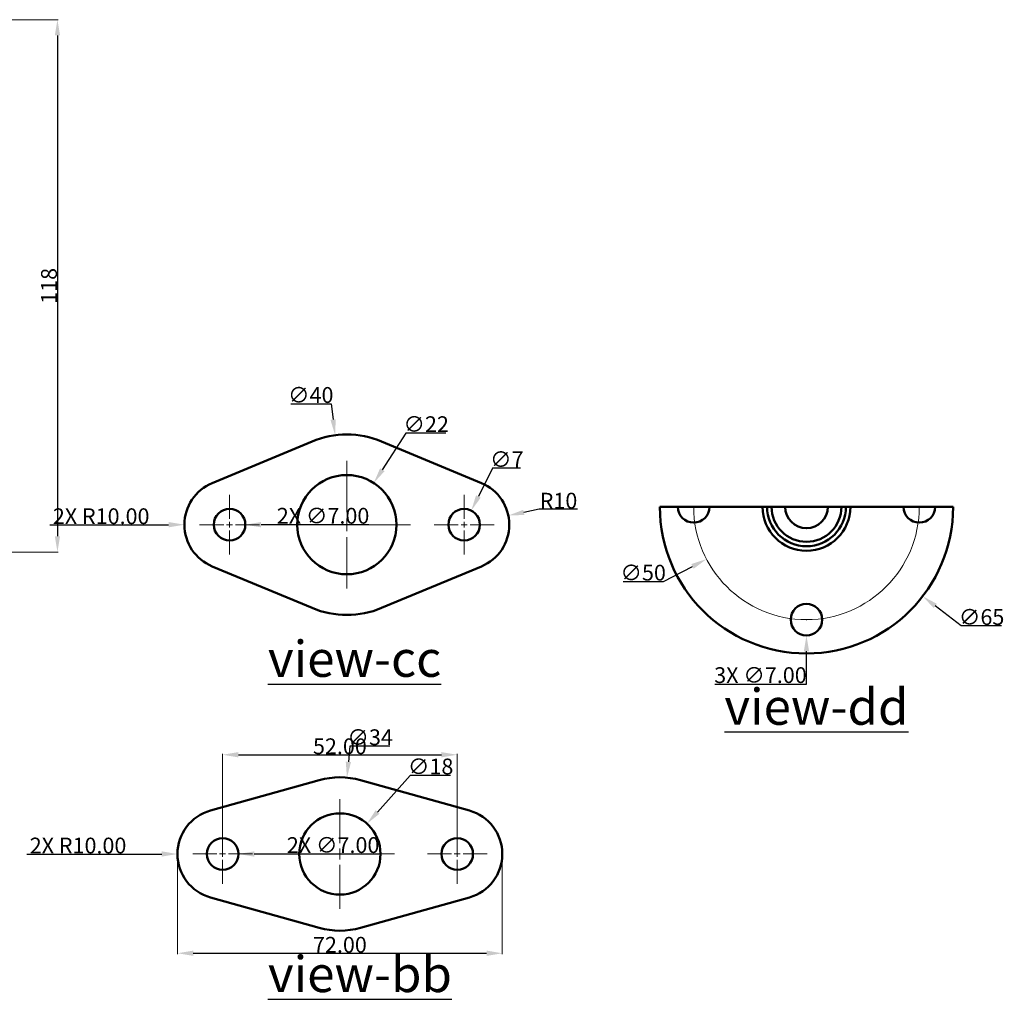
# Model space of a CAD drawing. Units: millimetres. Extents: x 75 to 489, y 21 to 350.
# Tile 5 of 5: x 271 to 489, y 110 to 327. Entities that reach past the tile are written whole.
import ezdxf

# ---------------------------------------------------------------- set-up
doc = ezdxf.new("R2010")
doc.units = ezdxf.units.MM
doc.header["$MEASUREMENT"] = 0
doc.linetypes.add('CENTER', pattern=[50.8, 31.75, -6.35, 6.35, -6.35])
for name, color, linetype, lineweight in [('M-CNTR', 1, 'CENTER', 18), ('M-CONS', 9, 'Continuous', 13), ('M-DIMS', 2, 'Continuous', 25), ('M-OUTL', 7, 'Continuous', 50), ('M-TEXT', 7, 'Continuous', 25)]:
    doc.layers.add(name, color=color, linetype=linetype, lineweight=lineweight)
doc.styles.get("Standard").update_dxf_attribs({"font": 'arial.ttf'})
doc.dimstyles.get("Standard").update_dxf_attribs({"dimtxt": 3.5, "dimasz": 3.5, "dimexe": 0.18, "dimexo": 0.0625, "dimgap": 0.09, "dimtad": 1, "dimtoh": 1, "dimdec": 0, "dimzin": 0, "dimdsep": 46, "dimtxsty": 'Standard', "dimcen": 0.09, "dimclrd": 2, "dimclre": 251, "dimadec": 0, "dimazin": 0, "dimtfac": 1, "dimtdec": 0, "dimtofl": 0, "dimtmove": 0, "dimatfit": 3, "dimfxl": 1, "dimtolj": 1, "dimtzin": 0, "dimlwe": 5, "dimarcsym": 0})

# ---------------------------------------------------------------- blocks, each defined once
blk = doc.blocks.new('*U1')
at = {"layer": 'M-CNTR', "color": 0, "transparency": 16777216}
for p, q in [((0, 1.3), (0, 6.62)), ((-6.62, 0), (-1.3, 0)), ((1.3, 0), (6.62, 0)), ((0, -6.62), (0, -1.3))]:
    blk.add_line(p, q, dxfattribs=at)
at = {"layer": 'M-CNTR', "color": 0, "linetype": 'Continuous', "transparency": 16777216}
for p, q in [((-0.65, 0), (0.65, 0)), ((0, -0.65), (0, 0.65))]:
    blk.add_line(p, q, dxfattribs=at)
blk = doc.blocks.new('*U2')
at = {"layer": 'M-CNTR', "color": 0, "transparency": 16777216}
for p, q in [((0, 1.3), (0, 6.62)), ((-6.62, 0), (-1.3, 0)), ((1.3, 0), (6.62, 0)), ((0, -6.62), (0, -1.3))]:
    blk.add_line(p, q, dxfattribs=at)
at = {"layer": 'M-CNTR', "color": 0, "linetype": 'Continuous', "transparency": 16777216}
for p, q in [((-0.65, 0), (0.65, 0)), ((0, -0.65), (0, 0.65))]:
    blk.add_line(p, q, dxfattribs=at)
blk = doc.blocks.new('*U3')
at = {"layer": 'M-CNTR', "color": 0, "transparency": 16777216}
for p, q in [((0, 2.8), (0, 14.12)), ((-14.12, 0), (-2.8, 0)), ((2.8, 0), (14.12, 0)), ((0, -14.12), (0, -2.8))]:
    blk.add_line(p, q, dxfattribs=at)
at = {"layer": 'M-CNTR', "color": 0, "linetype": 'Continuous', "transparency": 16777216}
for p, q in [((-1.4, 0), (1.4, 0)), ((0, -1.4), (0, 1.4))]:
    blk.add_line(p, q, dxfattribs=at)
blk = doc.blocks.new('*D4')
at = {"layer": 'Defpoints', "color": 0, "transparency": 16777216}
for p in [(349.6, 224.66), (337.68, 206.17)]:
    blk.add_point(p, dxfattribs=at)
at = {"layer": 'M-DIMS', "color": 0, "lineweight": -2, "transparency": 16777216}
for p, q in [((356.74, 235.71), (351.5, 227.6)), ((365.61, 235.71), (356.74, 235.71))]:
    blk.add_line(p, q, dxfattribs=at)
at = {"layer": 'M-DIMS', "color": 0, "lineweight": 5, "transparency": 16777216}
for p, q in [((343.55, 215.41), (343.73, 215.41)), ((343.64, 215.32), (343.64, 215.5))]:
    blk.add_line(p, q, dxfattribs=at)
at = {"layer": 'M-DIMS', "color": 0, "transparency": 16777216}
blk.add_solid([(351.01, 227.91), (351.99, 227.28), (349.6, 224.66)], dxfattribs=at)
at = {"layer": 'M-DIMS', "color": 0, "transparency": 16777216, "insert": (361.22, 237.69), "char_height": 3.5, "attachment_point": 5}
blk.add_mtext('\\A1;∅22', dxfattribs=at)
blk = doc.blocks.new('*D5')
at = {"layer": 'Defpoints', "color": 0, "transparency": 16777216}
for p in [(341.05, 235.24), (346.23, 195.58)]:
    blk.add_point(p, dxfattribs=at)
at = {"layer": 'M-DIMS', "color": 0, "lineweight": -2, "transparency": 16777216}
for p, q in [((331.24, 242.18), (340.14, 242.18)), ((340.14, 242.18), (340.59, 238.71))]:
    blk.add_line(p, q, dxfattribs=at)
at = {"layer": 'M-DIMS', "color": 0, "lineweight": 5, "transparency": 16777216}
for p, q in [((343.55, 215.41), (343.73, 215.41)), ((343.64, 215.32), (343.64, 215.5))]:
    blk.add_line(p, q, dxfattribs=at)
at = {"layer": 'M-DIMS', "color": 0, "transparency": 16777216}
blk.add_solid([(341.17, 238.79), (340.01, 238.64), (341.05, 235.24)], dxfattribs=at)
at = {"layer": 'M-DIMS', "color": 0, "transparency": 16777216, "insert": (335.64, 244.16), "char_height": 3.5, "attachment_point": 5}
blk.add_mtext('\\A1;∅40', dxfattribs=at)
blk = doc.blocks.new('*D6')
at = {"layer": 'Defpoints', "color": 0, "transparency": 16777216}
for p in [(371.22, 218.54), (368.06, 212.29)]:
    blk.add_point(p, dxfattribs=at)
at = {"layer": 'M-DIMS', "color": 0, "lineweight": -2, "transparency": 16777216}
for p, q in [((375.95, 227.93), (372.79, 221.66)), ((382.14, 227.93), (375.95, 227.93))]:
    blk.add_line(p, q, dxfattribs=at)
at = {"layer": 'M-DIMS', "color": 0, "lineweight": 5, "transparency": 16777216}
for p, q in [((369.55, 215.41), (369.73, 215.41)), ((369.64, 215.32), (369.64, 215.5))]:
    blk.add_line(p, q, dxfattribs=at)
at = {"layer": 'M-DIMS', "color": 0, "transparency": 16777216}
blk.add_solid([(372.27, 221.93), (373.31, 221.4), (371.22, 218.54)], dxfattribs=at)
at = {"layer": 'M-DIMS', "color": 0, "transparency": 16777216, "insert": (379.09, 229.9), "char_height": 3.5, "attachment_point": 5}
blk.add_mtext('\\A1;∅7', dxfattribs=at)
blk = doc.blocks.new('*D7')
at = {"layer": 'Defpoints', "color": 0, "transparency": 16777216}
for p in [(379.43, 217.44), (369.64, 215.41)]:
    blk.add_point(p, dxfattribs=at)
at = {"layer": 'M-DIMS', "color": 0, "lineweight": -2, "transparency": 16777216}
for p, q in [((386.29, 218.85), (382.86, 218.14)), ((394.73, 218.85), (386.29, 218.85))]:
    blk.add_line(p, q, dxfattribs=at)
at = {"layer": 'M-DIMS', "color": 0, "lineweight": 5, "transparency": 16777216}
for p, q in [((369.55, 215.41), (369.73, 215.41)), ((369.64, 215.32), (369.64, 215.5))]:
    blk.add_line(p, q, dxfattribs=at)
at = {"layer": 'M-DIMS', "color": 0, "transparency": 16777216}
blk.add_solid([(382.74, 218.71), (382.98, 217.57), (379.43, 217.44)], dxfattribs=at)
at = {"layer": 'M-DIMS', "color": 0, "transparency": 16777216, "insert": (390.55, 220.73), "char_height": 3.5, "attachment_point": 5}
blk.add_mtext('\\A1;R10', dxfattribs=at)
blk = doc.blocks.new('*U8')
at = {"layer": 'M-CNTR', "color": 0, "transparency": 16777216}
for p, q in [((0, 1.3), (0, 6.62)), ((-6.62, 0), (-1.3, 0)), ((1.3, 0), (6.62, 0)), ((0, -6.62), (0, -1.3))]:
    blk.add_line(p, q, dxfattribs=at)
at = {"layer": 'M-CNTR', "color": 0, "linetype": 'Continuous', "transparency": 16777216}
for p, q in [((-0.65, 0), (0.65, 0)), ((0, -0.65), (0, 0.65))]:
    blk.add_line(p, q, dxfattribs=at)
blk = doc.blocks.new('*U9')
at = {"layer": 'M-CNTR', "color": 0, "transparency": 16777216}
for p, q in [((0, 2.4), (0, 12.12)), ((-12.12, 0), (-2.4, 0)), ((2.4, 0), (12.12, 0)), ((0, -12.12), (0, -2.4))]:
    blk.add_line(p, q, dxfattribs=at)
at = {"layer": 'M-CNTR', "color": 0, "linetype": 'Continuous', "transparency": 16777216}
for p, q in [((-1.2, 0), (1.2, 0)), ((0, -1.2), (0, 1.2))]:
    blk.add_line(p, q, dxfattribs=at)
blk = doc.blocks.new('*U10')
at = {"layer": 'M-CNTR', "color": 0, "transparency": 16777216}
for p, q in [((0, 1.3), (0, 6.62)), ((-6.62, 0), (-1.3, 0)), ((1.3, 0), (6.62, 0)), ((0, -6.62), (0, -1.3))]:
    blk.add_line(p, q, dxfattribs=at)
at = {"layer": 'M-CNTR', "color": 0, "linetype": 'Continuous', "transparency": 16777216}
for p, q in [((-0.65, 0), (0.65, 0)), ((0, -0.65), (0, 0.65))]:
    blk.add_line(p, q, dxfattribs=at)
blk = doc.blocks.new('*D11')
at = {"layer": 'Defpoints', "color": 0, "transparency": 16777216}
for p in [(343.66, 159.35), (340.53, 125.5)]:
    blk.add_point(p, dxfattribs=at)
at = {"layer": 'M-DIMS', "color": 0, "lineweight": -2, "transparency": 16777216}
for p, q in [((344.31, 166.32), (343.98, 162.84)), ((353.2, 166.32), (344.31, 166.32))]:
    blk.add_line(p, q, dxfattribs=at)
at = {"layer": 'M-DIMS', "color": 0, "lineweight": 5, "transparency": 16777216}
for p, q in [((342.01, 142.42), (342.19, 142.42)), ((342.1, 142.33), (342.1, 142.51))]:
    blk.add_line(p, q, dxfattribs=at)
at = {"layer": 'M-DIMS', "color": 0, "transparency": 16777216}
blk.add_solid([(343.4, 162.89), (344.56, 162.78), (343.66, 159.35)], dxfattribs=at)
at = {"layer": 'M-DIMS', "color": 0, "transparency": 16777216, "insert": (348.8, 168.3), "char_height": 3.5, "attachment_point": 5}
blk.add_mtext('\\A1;∅34', dxfattribs=at)
blk = doc.blocks.new('*D12')
at = {"layer": 'Defpoints', "color": 0, "transparency": 16777216}
for p in [(348.1, 149.13), (336.09, 135.72)]:
    blk.add_point(p, dxfattribs=at)
at = {"layer": 'M-DIMS', "color": 0, "lineweight": -2, "transparency": 16777216}
for p, q in [((357.71, 159.84), (350.44, 151.73)), ((366.63, 159.84), (357.71, 159.84))]:
    blk.add_line(p, q, dxfattribs=at)
at = {"layer": 'M-DIMS', "color": 0, "lineweight": 5, "transparency": 16777216}
for p, q in [((342.01, 142.42), (342.19, 142.42)), ((342.1, 142.33), (342.1, 142.51))]:
    blk.add_line(p, q, dxfattribs=at)
at = {"layer": 'M-DIMS', "color": 0, "transparency": 16777216}
blk.add_solid([(350.01, 152.12), (350.87, 151.34), (348.1, 149.13)], dxfattribs=at)
at = {"layer": 'M-DIMS', "color": 0, "transparency": 16777216, "insert": (362.21, 161.82), "char_height": 3.5, "attachment_point": 5}
blk.add_mtext('\\A1;∅18', dxfattribs=at)
blk = doc.blocks.new('*D13')
at = {"layer": 'Defpoints', "color": 0, "transparency": 16777216}
for p in [(419.75, 239.19), (471.27, 199.55)]:
    blk.add_point(p, dxfattribs=at)
at = {"layer": 'M-DIMS', "color": 0, "lineweight": 5, "transparency": 16777216}
for p, q in [((445.42, 219.37), (445.6, 219.37)), ((445.51, 219.28), (445.51, 219.46))]:
    blk.add_line(p, q, dxfattribs=at)
at = {"layer": 'M-DIMS', "color": 0, "lineweight": -2, "transparency": 16777216}
for p, q in [((479.8, 192.98), (474.04, 197.41)), ((488.74, 192.98), (479.8, 192.98))]:
    blk.add_line(p, q, dxfattribs=at)
at = {"layer": 'M-DIMS', "color": 0, "transparency": 16777216}
blk.add_solid([(474.4, 197.88), (473.69, 196.95), (471.27, 199.55)], dxfattribs=at)
at = {"layer": 'M-DIMS', "color": 0, "transparency": 16777216, "insert": (484.32, 194.95), "char_height": 3.5, "attachment_point": 5}
blk.add_mtext('\\A1;∅65', dxfattribs=at)
blk = doc.blocks.new('*D14')
at = {"layer": 'Defpoints', "color": 0, "transparency": 16777216}
for p in [(467.67, 230.94), (423.35, 207.79)]:
    blk.add_point(p, dxfattribs=at)
at = {"layer": 'M-DIMS', "color": 0, "lineweight": 5, "transparency": 16777216}
for p, q in [((445.42, 219.37), (445.6, 219.37)), ((445.51, 219.28), (445.51, 219.46))]:
    blk.add_line(p, q, dxfattribs=at)
at = {"layer": 'M-DIMS', "color": 0, "lineweight": -2, "transparency": 16777216}
for p, q in [((413.81, 202.8), (420.25, 206.17)), ((404.91, 202.8), (413.81, 202.8))]:
    blk.add_line(p, q, dxfattribs=at)
at = {"layer": 'M-DIMS', "color": 0, "transparency": 16777216}
blk.add_solid([(419.98, 206.69), (420.52, 205.65), (423.35, 207.79)], dxfattribs=at)
at = {"layer": 'M-DIMS', "color": 0, "transparency": 16777216, "insert": (409.31, 204.78), "char_height": 3.5, "attachment_point": 5}
blk.add_mtext('\\A1;∅50', dxfattribs=at)
blk = doc.blocks.new('*D35')
at = {"layer": 'Defpoints', "color": 0, "transparency": 16777216}
for p in [(220.88, 327.35), (259, 209.35), (279.5, 209.35)]:
    blk.add_point(p, dxfattribs=at)
at = {"layer": 'M-DIMS', "color": 0, "lineweight": 5, "transparency": 16777216}
for p, q in [((220.95, 327.35), (279.68, 327.35)), ((259.06, 209.35), (279.68, 209.35))]:
    blk.add_line(p, q, dxfattribs=at)
at = {"layer": 'M-DIMS', "color": 0, "lineweight": -2, "transparency": 16777216}
blk.add_line((279.5, 323.85), (279.5, 212.85), dxfattribs=at)
at = {"layer": 'M-DIMS', "color": 0, "transparency": 16777216}
for points in [[(278.92, 323.85), (280.08, 323.85), (279.5, 327.35)], [(278.92, 212.85), (280.08, 212.85), (279.5, 209.35)]]:
    blk.add_solid(points, dxfattribs=at)
at = {"layer": 'M-DIMS', "color": 0, "transparency": 16777216, "insert": (277.62, 268.35), "char_height": 3.5, "attachment_point": 5, "rotation": 90}
blk.add_mtext('\\A1;118', dxfattribs=at)
blk = doc.blocks.new('*D62')
at = {"layer": 'Defpoints', "color": 0, "transparency": 16777216}
for p in [(368.1, 164.42), (316.1, 142.42), (368.1, 142.42)]:
    blk.add_point(p, dxfattribs=at)
at = {"layer": 'M-DIMS', "color": 251, "lineweight": 5, "transparency": 16777216}
for p, q in [((316.1, 142.49), (316.1, 164.6)), ((368.1, 142.49), (368.1, 164.6))]:
    blk.add_line(p, q, dxfattribs=at)
at = {"layer": 'M-DIMS', "color": 2, "lineweight": -2, "transparency": 16777216}
blk.add_line((319.6, 164.42), (364.6, 164.42), dxfattribs=at)
at = {"layer": 'M-DIMS', "color": 2, "transparency": 16777216}
for points in [[(319.6, 165.01), (319.6, 163.84), (316.1, 164.42)], [(364.6, 165.01), (364.6, 163.84), (368.1, 164.42)]]:
    blk.add_solid(points, dxfattribs=at)
at = {"layer": 'M-DIMS', "color": 0, "transparency": 16777216, "insert": (342.1, 166.3), "char_height": 3.5, "attachment_point": 5}
blk.add_mtext('\\A1;52.00', dxfattribs=at)
blk = doc.blocks.new('*D63')
at = {"layer": 'Defpoints', "color": 0, "transparency": 16777216}
for p in [(306.1, 142.42), (378.1, 142.42), (378.1, 120.42)]:
    blk.add_point(p, dxfattribs=at)
at = {"layer": 'M-DIMS', "color": 251, "lineweight": 5, "transparency": 16777216}
for p, q in [((306.1, 142.36), (306.1, 120.24)), ((378.1, 142.36), (378.1, 120.24))]:
    blk.add_line(p, q, dxfattribs=at)
at = {"layer": 'M-DIMS', "color": 2, "lineweight": -2, "transparency": 16777216}
blk.add_line((309.6, 120.42), (374.6, 120.42), dxfattribs=at)
at = {"layer": 'M-DIMS', "color": 2, "transparency": 16777216}
for points in [[(309.6, 121.01), (309.6, 119.84), (306.1, 120.42)], [(374.6, 121.01), (374.6, 119.84), (378.1, 120.42)]]:
    blk.add_solid(points, dxfattribs=at)
at = {"layer": 'M-DIMS', "color": 0, "transparency": 16777216, "insert": (342.1, 122.3), "char_height": 3.5, "attachment_point": 5}
blk.add_mtext('\\A1;72.00', dxfattribs=at)
blk = doc.blocks.new('*D65')
at = {"layer": 'Defpoints', "color": 0, "transparency": 16777216}
for p in [(314.14, 215.41), (321.14, 215.41)]:
    blk.add_point(p, dxfattribs=at)
at = {"layer": 'M-DIMS', "color": 251, "lineweight": 5, "transparency": 16777216}
for p, q in [((317.55, 215.41), (317.73, 215.41)), ((317.64, 215.32), (317.64, 215.5))]:
    blk.add_line(p, q, dxfattribs=at)
at = {"layer": 'M-DIMS', "color": 2, "lineweight": -2, "transparency": 16777216}
for p, q in [((328.14, 215.41), (324.64, 215.41)), ((348.51, 215.41), (328.14, 215.41))]:
    blk.add_line(p, q, dxfattribs=at)
at = {"layer": 'M-DIMS', "color": 2, "transparency": 16777216}
blk.add_solid([(324.64, 216), (324.64, 214.83), (321.14, 215.41)], dxfattribs=at)
at = {"layer": 'M-DIMS', "color": 0, "transparency": 16777216, "insert": (338.37, 217.39), "char_height": 3.5, "attachment_point": 5}
blk.add_mtext('\\A1;2X ∅7.00', dxfattribs=at)
blk = doc.blocks.new('*D66')
at = {"layer": 'Defpoints', "color": 0, "transparency": 16777216}
for p in [(307.64, 215.41), (317.64, 215.41)]:
    blk.add_point(p, dxfattribs=at)
at = {"layer": 'M-DIMS', "color": 2, "lineweight": -2, "transparency": 16777216}
for p, q in [((277.82, 215.41), (300.64, 215.41)), ((300.64, 215.41), (304.14, 215.41))]:
    blk.add_line(p, q, dxfattribs=at)
at = {"layer": 'M-DIMS', "color": 251, "lineweight": 5, "transparency": 16777216}
for p, q in [((317.55, 215.41), (317.73, 215.41)), ((317.64, 215.32), (317.64, 215.5))]:
    blk.add_line(p, q, dxfattribs=at)
at = {"layer": 'M-DIMS', "color": 2, "transparency": 16777216}
blk.add_solid([(304.14, 216), (304.14, 214.83), (307.64, 215.41)], dxfattribs=at)
at = {"layer": 'M-DIMS', "color": 0, "transparency": 16777216, "insert": (289.19, 217.29), "char_height": 3.5, "attachment_point": 5}
blk.add_mtext('\\A1;2X R10.00', dxfattribs=at)
blk = doc.blocks.new('*D67')
at = {"layer": 'Defpoints', "color": 0, "transparency": 16777216}
for p in [(312.6, 142.42), (319.6, 142.42)]:
    blk.add_point(p, dxfattribs=at)
at = {"layer": 'M-DIMS', "color": 251, "lineweight": 5, "transparency": 16777216}
for p, q in [((316.01, 142.42), (316.19, 142.42)), ((316.1, 142.33), (316.1, 142.51))]:
    blk.add_line(p, q, dxfattribs=at)
at = {"layer": 'M-DIMS', "color": 2, "lineweight": -2, "transparency": 16777216}
for p, q in [((330.37, 142.42), (323.1, 142.42)), ((350.74, 142.42), (330.37, 142.42))]:
    blk.add_line(p, q, dxfattribs=at)
at = {"layer": 'M-DIMS', "color": 2, "transparency": 16777216}
blk.add_solid([(323.1, 143.01), (323.1, 141.84), (319.6, 142.42)], dxfattribs=at)
at = {"layer": 'M-DIMS', "color": 0, "transparency": 16777216, "insert": (340.6, 144.4), "char_height": 3.5, "attachment_point": 5}
blk.add_mtext('\\A1;2X ∅7.00', dxfattribs=at)
blk = doc.blocks.new('*D68')
at = {"layer": 'Defpoints', "color": 0, "transparency": 16777216}
for p in [(306.1, 142.42), (316.1, 142.42)]:
    blk.add_point(p, dxfattribs=at)
at = {"layer": 'M-DIMS', "color": 2, "lineweight": -2, "transparency": 16777216}
for p, q in [((272.71, 142.42), (295.52, 142.42)), ((295.52, 142.42), (302.6, 142.42))]:
    blk.add_line(p, q, dxfattribs=at)
at = {"layer": 'M-DIMS', "color": 251, "lineweight": 5, "transparency": 16777216}
for p, q in [((316.01, 142.42), (316.19, 142.42)), ((316.1, 142.33), (316.1, 142.51))]:
    blk.add_line(p, q, dxfattribs=at)
at = {"layer": 'M-DIMS', "color": 2, "transparency": 16777216}
blk.add_solid([(302.6, 143.01), (302.6, 141.84), (306.1, 142.42)], dxfattribs=at)
at = {"layer": 'M-DIMS', "color": 0, "transparency": 16777216, "insert": (284.07, 144.3), "char_height": 3.5, "attachment_point": 5}
blk.add_mtext('\\A1;2X R10.00', dxfattribs=at)
blk = doc.blocks.new('*D69')
at = {"layer": 'Defpoints', "color": 0, "transparency": 16777216}
for p in [(445.51, 197.87), (445.51, 190.87)]:
    blk.add_point(p, dxfattribs=at)
at = {"layer": 'M-DIMS', "color": 251, "lineweight": 5, "transparency": 16777216}
for p, q in [((445.42, 194.37), (445.6, 194.37)), ((445.51, 194.28), (445.51, 194.46))]:
    blk.add_line(p, q, dxfattribs=at)
at = {"layer": 'M-DIMS', "color": 2, "lineweight": -2, "transparency": 16777216}
for p, q in [((445.51, 180.1), (445.51, 187.37)), ((425.2, 180.1), (445.51, 180.1))]:
    blk.add_line(p, q, dxfattribs=at)
at = {"layer": 'M-DIMS', "color": 2, "transparency": 16777216}
blk.add_solid([(444.93, 187.37), (446.09, 187.37), (445.51, 190.87)], dxfattribs=at)
at = {"layer": 'M-DIMS', "color": 0, "transparency": 16777216, "insert": (435.31, 182.07), "char_height": 3.5, "attachment_point": 5}
blk.add_mtext('\\A1;3X ∅7.00', dxfattribs=at)

msp = doc.modelspace()

# ---------------------------------------------------------------- linework, layer by layer
at = {"layer": 'M-CNTR', "ltscale": 5}
msp.add_arc((445.509, 219.367), 25, 180, 0, dxfattribs=at)
at = {"layer": 'M-CONS'}
msp.add_point((445.509, 219.367), dxfattribs=at)
at = {"layer": 'M-OUTL'}
for p, q in [((313.793, 224.644), (335.947, 233.874)), ((373.486, 224.644), (351.332, 233.874)), ((413.009, 219.367), (478.009, 219.367)), ((313.793, 206.182), (335.947, 196.951)), ((373.486, 206.182), (351.332, 196.951)), ((313.405, 152.055), (337.521, 158.796)), ((370.79, 152.055), (346.675, 158.796)), ((313.405, 132.793), (337.521, 126.052)), ((370.79, 132.793), (346.675, 126.052))]:
    msp.add_line(p, q, dxfattribs=at)
for centre, radius in [((343.639, 215.413), 11), ((317.639, 215.413), 3.5), ((369.639, 215.413), 3.5), ((445.509, 194.367), 3.5), ((342.098, 142.424), 9), ((316.098, 142.424), 3.5), ((368.098, 142.424), 3.5)]:
    msp.add_circle(centre, radius, dxfattribs=at)
for centre, radius, start, end in [((343.639, 215.413), 20, 67.38014, 112.61986), ((317.639, 215.413), 10, 112.61986, 247.38014), ((369.639, 215.413), 10, 292.61986, 67.38014), ((445.509, 219.367), 32.5, 180, 0), ((420.509, 219.367), 3.5, 180, 0), ((445.509, 219.367), 9.738, 180, 0), ((445.509, 219.367), 8.738, 180, 0), ((445.509, 219.367), 7.738, 180, 0), ((445.509, 219.367), 4.738, 180, 0), ((470.509, 219.367), 3.5, 180, 0), ((343.639, 215.413), 20, 247.38014, 292.61986), ((342.098, 142.424), 17, 74.3815, 105.6185), ((316.098, 142.424), 10, 105.6185, 254.3815), ((368.098, 142.424), 10, 285.6185, 74.3815), ((342.098, 142.424), 17, 254.3815, 285.6185)]:
    msp.add_arc(centre, radius, start, end, dxfattribs=at)

# ---------------------------------------------------------------- block references
at = {"layer": 'M-CNTR'}
for name, p in [('*U3', (343.639, 215.413)), ('*U1', (317.639, 215.413)), ('*U2', (369.639, 215.413)), ('*U9', (342.098, 142.424)), ('*U10', (316.098, 142.424)), ('*U8', (368.098, 142.424))]:
    msp.add_blockref(name, p, dxfattribs=at)

# ---------------------------------------------------------------- texts
at = {"layer": 'M-TEXT', "char_height": 8, "attachment_point": 1}
for s, insert in [('{\\Lview-cc}', (326.161, 189.691)), ('{\\Lview-dd}', (427.316, 179.069)), ('{\\Lview-bb}', (326.161, 119.815))]:
    msp.add_mtext_dynamic_manual_height_columns(s, width=43.19704, gutter_width=1, heights=[0], dxfattribs=dict(at, insert=insert))

# ---------------------------------------------------------------- dimensions: what is measured, and where the dimension line sits
at = {"layer": 'M-DIMS'}
dim = msp.add_linear_dim(base=(279.5, 209.347), p1=(220.885, 327.347), p2=(259, 209.347), angle=90, dimstyle='Standard', override={"dimclrd": 0, "dimclre": 0, "dimclrt": 0}, dxfattribs=at)
dim.commit()
dim.dimension.update_dxf_attribs({"geometry": '*D35', "text_midpoint": (277.623, 268.347)})
for p1, p2, picture, middle in [((346.233, 195.582), (341.045, 235.244), '*D5', (335.643, 244.16)), ((419.752, 239.186), (471.267, 199.547), '*D13', (484.316, 194.955)), ((467.667, 230.944), (423.352, 207.789), '*D14', (409.311, 204.777)), ((340.534, 125.496), (343.662, 159.352), '*D11', (348.799, 168.297))]:
    dim = msp.add_diameter_dim_2p(p1=p1, p2=p2, dimstyle='Standard', override={"dimclrd": 0, "dimclre": 0, "dimclrt": 0}, dxfattribs=at)
    dim.commit()
    dim.dimension.update_dxf_attribs({"geometry": picture, "text_midpoint": middle})
for p1, p2, picture, middle in [((337.676, 206.17), (349.603, 224.656), '*D4', (361.219, 235.714)), ((368.063, 212.288), (371.216, 218.538), '*D6', (379.092, 227.925)), ((336.091, 135.722), (348.104, 149.127), '*D12', (362.212, 159.842))]:
    dim = msp.add_diameter_dim_2p(p1=p1, p2=p2, dimstyle='Standard', override={"dimclrd": 0, "dimclre": 0, "dimclrt": 0}, dxfattribs=at)
    dim.commit()
    dim.dimension.update_dxf_attribs({"geometry": picture, "text_midpoint": middle, "dimtype": 163})
for p1, p2, picture, middle in [((314.139, 215.413), (321.139, 215.413), '*D65', (328.139, 215.413)), ((312.598, 142.424), (319.598, 142.424), '*D67', (330.368, 142.424))]:
    dim = msp.add_diameter_dim_2p(p1=p1, p2=p2, text='2X <>', dimstyle='Standard', override={"dimdec": 2, "dimlfac": 1, "dimrnd": 0, "dimzin": 0, "dimdsep": 46, "dimlunit": 2}, dxfattribs=at)
    dim.commit()
    dim.dimension.update_dxf_attribs({"geometry": picture, "text_midpoint": middle})
dim = msp.add_radius_dim(center=(369.639, 215.413), mpoint=(379.433, 217.435), dimstyle='Standard', override={"dimclrd": 0, "dimclre": 0, "dimclrt": 0}, dxfattribs=at)
dim.commit()
dim.dimension.update_dxf_attribs({"geometry": '*D7', "text_midpoint": (390.554, 220.728)})
for center, mpoint, picture, middle in [((317.639, 215.413), (307.639, 215.413), '*D66', (289.185, 217.29)), ((316.098, 142.424), (306.098, 142.424), '*D68', (284.069, 144.301))]:
    dim = msp.add_radius_dim(center=center, mpoint=mpoint, text='2X <>', dimstyle='Standard', override={"dimdec": 2, "dimlfac": 1, "dimrnd": 0, "dimzin": 0, "dimdsep": 46, "dimlunit": 2}, dxfattribs=at)
    dim.commit()
    dim.dimension.update_dxf_attribs({"geometry": picture, "text_midpoint": middle})
dim = msp.add_diameter_dim_2p(p1=(445.51, 197.867), p2=(445.509, 190.867), text='3X <>', dimstyle='Standard', override={"dimdec": 2, "dimlfac": 1, "dimrnd": 0, "dimzin": 0, "dimdsep": 46, "dimlunit": 2}, dxfattribs=at)
dim.commit()
dim.dimension.update_dxf_attribs({"geometry": '*D69', "text_midpoint": (435.308, 180.097), "dimtype": 163})
for base, p1, p2, picture, middle in [((368.098, 164.424), (316.098, 142.424), (368.098, 142.424), '*D62', (342.098, 166.301)), ((378.098, 120.424), (306.098, 142.424), (378.098, 142.424), '*D63', (342.098, 122.301))]:
    dim = msp.add_linear_dim(base=base, p1=p1, p2=p2, dimstyle='Standard', override={"dimdec": 2, "dimlfac": 1, "dimrnd": 0, "dimzin": 0, "dimdsep": 46, "dimlunit": 2}, dxfattribs=at)
    dim.commit()
    dim.dimension.update_dxf_attribs({"geometry": picture, "text_midpoint": middle})

doc.saveas('drawing.dxf')
